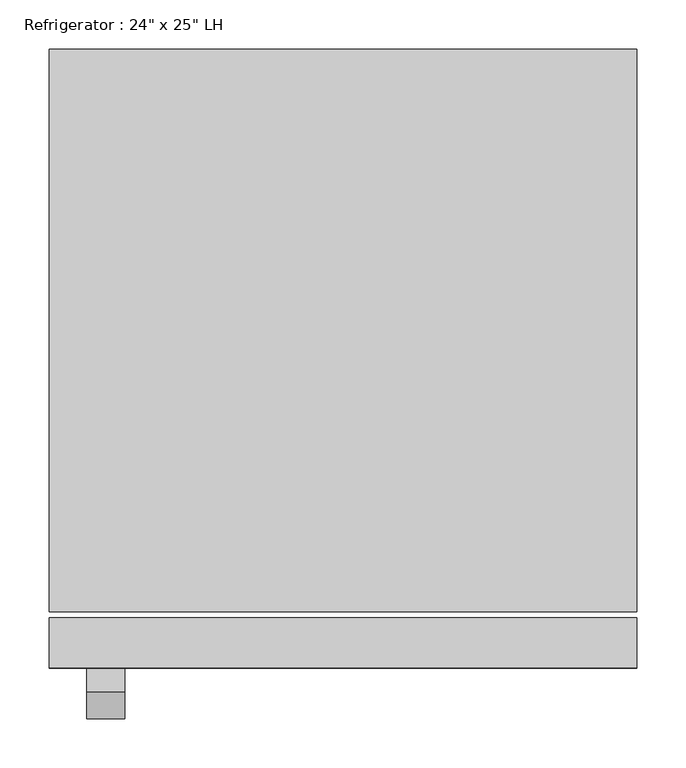
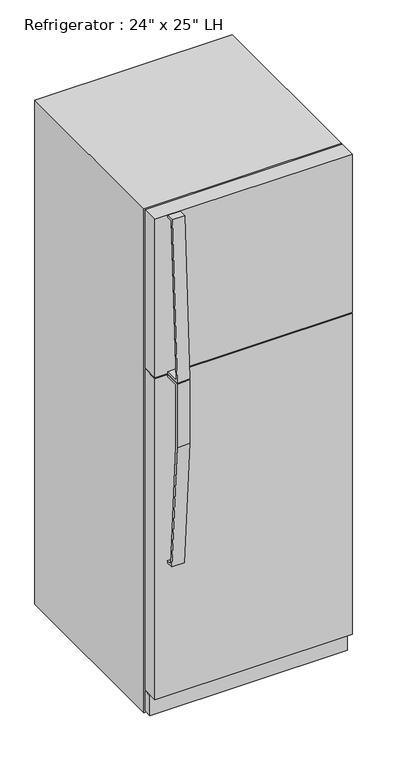
"""IFC4 building model written with IfcOpenShell, lengths in millimetres: proxy geometry."""

from ifc_helpers import new_model, si_unit, frame, origin, origin_with_axes, place, context, project, spatial, polyline, outline, extrude, source, transform, mapped, element, save


def proxy_c523a7b7(model_context):
    return source(origin(), model_context, "Body", "SweptSolid", [
        extrude(outline(polyline([(-329.0010285, 1096.9625), (-373.4510285, 1096.9625), (-373.4510285, 900.3342469), (-345.9723987, 507.3715334), (-329.0010285, 507.3715334), (-329.0010285, 501.0370017), (-351.8949512, 501.0370017), (-379.8010285, 900.1125), (-379.8010285, 1103.3125), (-329.0010285, 1103.3125), (-329.0010285, 1096.9625)])), frame((-260.35, 0.0, 0.0), z_axis=(1.0, 0.0, 0.0), x_axis=(0.0, 1.0, 0.0)), (0.0, 0.0, 1.0), 38.4332978),
        extrude(outline(polyline([(-353.839413, 1612.9), (-329.7780855, 1612.9), (-329.7780855, 1606.55), (-348.6263449, 1606.55), (-374.5007207, 1112.8375), (-329.7780855, 1112.8375), (-329.7780855, 1106.4875), (-380.3793675, 1106.4875), (-353.839413, 1612.9)])), frame((-260.35, 0.0, 0.0), z_axis=(1.0, 0.0, 0.0), x_axis=(0.0, 1.0, 0.0)), (0.0, 0.0, 1.0), 38.4332978),
        extrude(outline(polyline([(298.45, -278.2010285), (298.45, -303.6010285), (-298.45, -303.6010285), (-298.45, -278.2010285), (298.45, -278.2010285)])), frame((0.0, 0.0, 9.3816357), z_axis=(0.0, 0.0, 1.0), x_axis=(1.0, 0.0, 0.0)), (0.0, 0.0, 1.0), 63.5),
        extrude(outline(polyline([(298.45, -278.2010285), (298.45, -329.0010285), (-298.45, -329.0010285), (-298.45, -278.2010285), (298.45, -278.2010285)])), frame((0.0, 0.0, 76.2), z_axis=(0.0, 0.0, 1.0), x_axis=(1.0, 0.0, 0.0)), (0.0, 0.0, 1.0), 1027.1125),
        extrude(outline(polyline([(298.45, -278.2010285), (298.45, -329.0010285), (-298.45, -329.0010285), (-298.45, -278.2010285), (298.45, -278.2010285)])), frame((0.0, 0.0, 1106.4875), z_axis=(0.0, 0.0, 1.0), x_axis=(1.0, 0.0, 0.0)), (0.0, 0.0, 1.0), 506.4125),
        extrude(outline(polyline([(298.45, 299.6489715), (298.45, -271.8510285), (-298.45, -271.8510285), (-298.45, 299.6489715), (298.45, 299.6489715)])), origin_with_axes(), (0.0, 0.0, 1.0), 1612.9),
    ])


if __name__ == "__main__":
    model = new_model("IFC4")
    model_context = context("Model", 3, world=origin())
    ifc_project = project(units=[si_unit("LENGTHUNIT", "METRE", prefix="MILLI")], contexts=[model_context])
    site = spatial("IfcSite", under=ifc_project)
    building = spatial("IfcBuilding", under=site)
    placement = place(None, origin())
    proxy_shape = proxy_c523a7b7(model_context)
    element("IfcBuildingElementProxy", 1, Name="Refrigerator : 24\" x 25\" LH", ObjectType="Refrigerator : 24\" x 25\" LH", at=placement, inside=building, context=model_context, shape_type="MappedRepresentation", body=[
        mapped(proxy_shape, transform((0.0, 0.0, 0.0), x_axis=(1.0, 0.0, 0.0), y_axis=(0.0, 1.0, 0.0), z_axis=(0.0, 0.0, 1.0))),
    ])
    save(model, "model.ifc")

# Revit data of these elements
# Type "Refrigerator : 24\" x 25\" LH"
#   Label = "REF."
#   Assembly Code = "E1090400"
#   Depth = 2' - 0 3/4"
#   Handle = 0' - 1 1/2"
#   Height = 5' - 3 1/2"
#   Rear Clearance = 0' - 2"
#   Top Door Height = 1' - 8"
#   Width = 1' - 11 1/2"
#   Material = Steel, Paint Finish, Ivory, Glossy
#   Default Elevation = 0
# Element 1 (IfcBuildingElementProxy, "Refrigerator : 24\" x 25\" LH")
#   Materials on its faces: "Steel, Paint Finish, Ivory, Glossy", "Steel, Chrome Plated"
# Materials
#   "Steel, Paint Finish, Ivory, Glossy": class "Metal", colour RGB 247 247 239, transparency 0, Description = "Steel, paint finish, ivory, glossy", Cost = 0
#   "Steel, Chrome Plated": class "Metal", colour RGB 17 17 17, transparency 0, Description = "Chromiuim plated steel", Cost = 0
